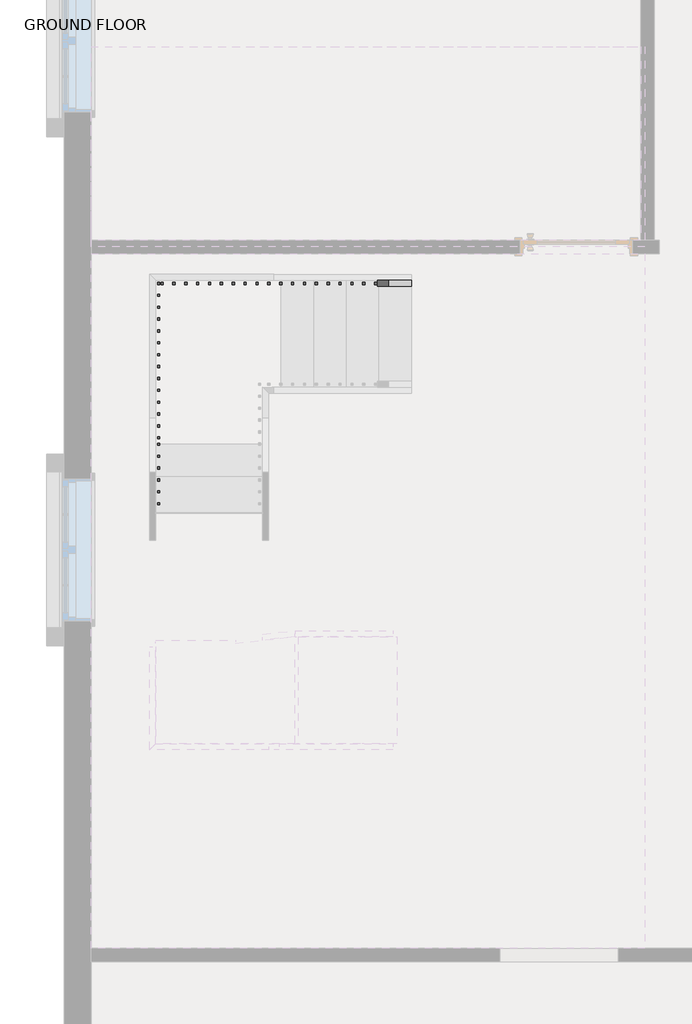
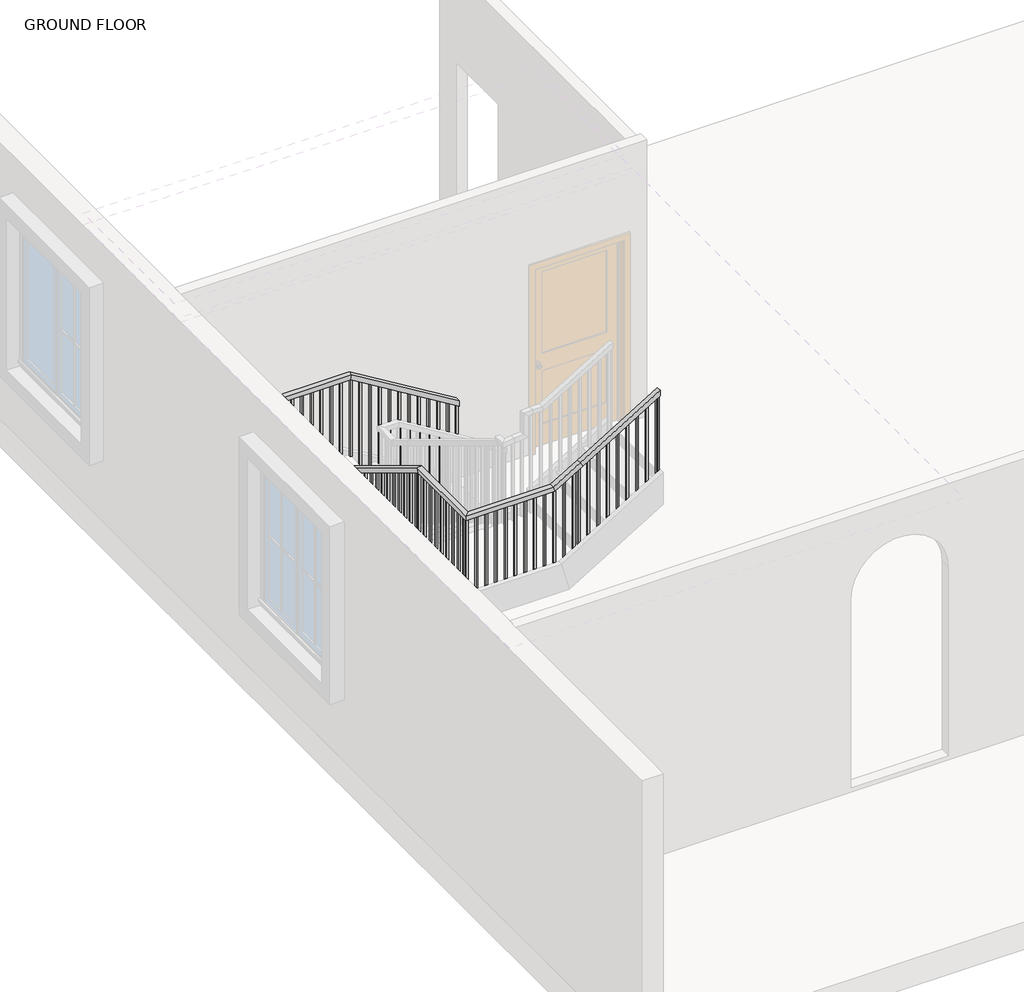
# One storey, part 2 of 4: 1 railing.
"""IFC4 building model written with IfcOpenShell, lengths in millimetres."""

from ifc_helpers import new_model, si_unit, frame, origin, place, context, project, spatial, polyline, outline, extrude, faceted_brep, element, save

model = new_model("IFC4")

# Units and contexts
model_context = context("Model", 3, world=origin())
ifc_project = project(units=[si_unit("LENGTHUNIT", "METRE", prefix="MILLI")], contexts=[model_context])

# Site, building, storey
site = spatial("IfcSite", under=ifc_project)
building = spatial("IfcBuilding", under=site)
storey = spatial("IfcBuildingStorey", under=building, Name="GROUND FLOOR", Elevation=304.8)

# Railing
placement = place(None, origin())
element("IfcRailing", 1, ObjectType="Handrail - Rectangular", at=placement, inside=storey, context=model_context, shape_type="SolidModel", body=[
    faceted_brep([(-9079.7156858, 994.3115003, 1388.5333333), (-9079.7156858, 994.3115003, 1329.1318731), (-9079.7156858, 1045.1115003, 1329.1318731), (-9079.7156858, 1045.1115003, 1388.5333333), (-10197.3156858, 994.3115003, 2065.8666667), (-10211.5080953, 994.3115003, 2015.0666667), (-10211.5080953, 1045.1115003, 2015.0666667), (-10197.3156858, 1045.1115003, 2065.8666667), (-11217.3522729, 994.3115003, 2065.8666667), (-11217.3522729, 994.3115003, 2015.0666667), (-11268.1522729, 1045.1115003, 2015.0666667), (-11268.1522729, 1045.1115003, 2065.8666667), (-11217.3522729, -76.9993654, 2065.8666667), (-11217.3522729, -91.1917748, 2015.0666667), (-11268.1522729, -91.1917748, 2015.0666667), (-11268.1522729, -76.9993654, 2065.8666667), (-11217.3522729, -356.3993654, 2235.2), (-11217.3522729, -382.7290926, 2191.7559502), (-11268.1522729, -382.7290926, 2191.7559502), (-11268.1522729, -356.3993654, 2235.2), (-11217.3522729, -2032.7993654, 3251.2), (-11217.3522729, -2046.9917748, 3200.4), (-11268.1522729, -2046.9917748, 3200.4), (-11268.1522729, -2032.7993654, 3251.2), (-11217.3522729, -2865.2844117, 3251.2), (-11217.3522729, -2865.2844117, 3200.4), (-11268.1522729, -2916.0844117, 3200.4), (-11268.1522729, -2916.0844117, 3251.2), (-10353.7522729, -2865.2844117, 3251.2), (-10339.5598635, -2865.2844117, 3200.4), (-10339.5598635, -2916.0844117, 3200.4), (-10353.7522729, -2916.0844117, 3251.2), (-10074.3522729, -2865.2844117, 3420.5333333), (-10048.0225457, -2865.2844117, 3377.0892835), (-10048.0225457, -2916.0844117, 3377.0892835), (-10074.3522729, -2916.0844117, 3420.5333333), (-9236.1522729, -2865.2844117, 3928.5333333), (-9236.1522729, -2916.0844117, 3928.5333333), (-9236.1522729, -2916.0844117, 3869.1318731), (-9236.1522729, -2865.2844117, 3869.1318731)], [[[0, 1, 2, 3]], [[1, 0, 4, 5]], [[2, 1, 5, 6]], [[3, 2, 6, 7]], [[0, 3, 7, 4]], [[5, 4, 8, 9]], [[6, 5, 9, 10]], [[7, 6, 10, 11]], [[4, 7, 11, 8]], [[9, 8, 12, 13]], [[10, 9, 13, 14]], [[11, 10, 14, 15]], [[8, 11, 15, 12]], [[13, 12, 16, 17]], [[14, 13, 17, 18]], [[15, 14, 18, 19]], [[12, 15, 19, 16]], [[17, 16, 20, 21]], [[18, 17, 21, 22]], [[19, 18, 22, 23]], [[16, 19, 23, 20]], [[21, 20, 24, 25]], [[22, 21, 25, 26]], [[23, 22, 26, 27]], [[20, 23, 27, 24]], [[25, 24, 28, 29]], [[26, 25, 29, 30]], [[27, 26, 30, 31]], [[24, 27, 31, 28]], [[29, 28, 32, 33]], [[30, 29, 33, 34]], [[31, 30, 34, 35]], [[28, 31, 35, 32]], [[36, 37, 38, 39]], [[33, 32, 36, 39]], [[34, 33, 39, 38]], [[35, 34, 38, 37]], [[32, 35, 37, 36]]]),
    extrude(outline(polyline([(3859.510661, -9252.0272729), (3847.9652064, -9271.0772729), (2844.8, -9271.0772729), (2844.8, -9252.0272729), (3859.510661, -9252.0272729)])), frame((0.0, -2900.2094117, 0.0), z_axis=(0.0, 1.0, 0.0), x_axis=(0.0, 0.0, 1.0)), (0.0, 0.0, 1.0), 19.05),
    extrude(outline(polyline([(3797.9349034, -9353.6272729), (3786.3894488, -9372.6772729), (2844.8, -9372.6772729), (2844.8, -9353.6272729), (3797.9349034, -9353.6272729)])), frame((0.0, -2900.2094117, 0.0), z_axis=(0.0, 1.0, 0.0), x_axis=(0.0, 0.0, 1.0)), (0.0, 0.0, 1.0), 19.05),
    extrude(outline(polyline([(3736.3591458, -9455.2272729), (3724.8136913, -9474.2772729), (2844.8, -9474.2772729), (2844.8, -9455.2272729), (3736.3591458, -9455.2272729)])), frame((0.0, -2900.2094117, 0.0), z_axis=(0.0, 1.0, 0.0), x_axis=(0.0, 0.0, 1.0)), (0.0, 0.0, 1.0), 19.05),
    extrude(outline(polyline([(3674.7833882, -9556.8272729), (3663.2379337, -9575.8772729), (2675.4666667, -9575.8772729), (2675.4666667, -9556.8272729), (3674.7833882, -9556.8272729)])), frame((0.0, -2900.2094117, 0.0), z_axis=(0.0, 1.0, 0.0), x_axis=(0.0, 0.0, 1.0)), (0.0, 0.0, 1.0), 19.05),
    extrude(outline(polyline([(3613.2076307, -9658.4272729), (3601.6621761, -9677.4772729), (2675.4666667, -9677.4772729), (2675.4666667, -9658.4272729), (3613.2076307, -9658.4272729)])), frame((0.0, -2900.2094117, 0.0), z_axis=(0.0, 1.0, 0.0), x_axis=(0.0, 0.0, 1.0)), (0.0, 0.0, 1.0), 19.05),
    extrude(outline(polyline([(3551.6960801, -9760.0272729), (3540.0063073, -9779.0772729), (2675.4666667, -9779.0772729), (2675.4666667, -9760.0272729), (3551.6960801, -9760.0272729)])), frame((0.0, -2900.2094117, 0.0), z_axis=(0.0, 1.0, 0.0), x_axis=(0.0, 0.0, 1.0)), (0.0, 0.0, 1.0), 19.05),
    extrude(outline(polyline([(3490.0561155, -9861.6272729), (3478.510661, -9880.6772729), (2506.1333333, -9880.6772729), (2506.1333333, -9861.6272729), (3490.0561155, -9861.6272729)])), frame((0.0, -2900.2094117, 0.0), z_axis=(0.0, 1.0, 0.0), x_axis=(0.0, 0.0, 1.0)), (0.0, 0.0, 1.0), 19.05),
    extrude(outline(polyline([(3428.4803579, -9963.2272729), (3416.9349034, -9982.2772729), (2506.1333333, -9982.2772729), (2506.1333333, -9963.2272729), (3428.4803579, -9963.2272729)])), frame((0.0, -2900.2094117, 0.0), z_axis=(0.0, 1.0, 0.0), x_axis=(0.0, 0.0, 1.0)), (0.0, 0.0, 1.0), 19.05),
    extrude(outline(polyline([(3336.1167216, -10115.6272729), (3324.571267, -10134.6772729), (2336.8, -10134.6772729), (2336.8, -10115.6272729), (3336.1167216, -10115.6272729)])), frame((0.0, -2900.2094117, 0.0), z_axis=(0.0, 1.0, 0.0), x_axis=(0.0, 0.0, 1.0)), (0.0, 0.0, 1.0), 19.05),
    extrude(outline(polyline([(3274.540964, -10217.2272729), (3262.9955094, -10236.2772729), (2336.8, -10236.2772729), (2336.8, -10217.2272729), (3274.540964, -10217.2272729)])), frame((0.0, -2900.2094117, 0.0), z_axis=(0.0, 1.0, 0.0), x_axis=(0.0, 0.0, 1.0)), (0.0, 0.0, 1.0), 19.05),
    extrude(outline(polyline([(3213.0294134, -10318.8272729), (3201.3396407, -10337.8772729), (2336.8, -10337.8772729), (2336.8, -10318.8272729), (3213.0294134, -10318.8272729)])), frame((0.0, -2900.2094117, 0.0), z_axis=(0.0, 1.0, 0.0), x_axis=(0.0, 0.0, 1.0)), (0.0, 0.0, 1.0), 19.05),
    extrude(outline(polyline([(-10439.4772729, -2900.2094117), (-10439.4772729, -2881.1594117), (-10420.4272729, -2881.1594117), (-10420.4272729, -2900.2094117), (-10439.4772729, -2900.2094117)])), frame((0.0, 0.0, 2336.8), z_axis=(0.0, 0.0, 1.0), x_axis=(1.0, 0.0, 0.0)), (0.0, 0.0, 1.0), 863.6),
    extrude(outline(polyline([(-10541.0772729, -2900.2094117), (-10541.0772729, -2881.1594117), (-10522.0272729, -2881.1594117), (-10522.0272729, -2900.2094117), (-10541.0772729, -2900.2094117)])), frame((0.0, 0.0, 2336.8), z_axis=(0.0, 0.0, 1.0), x_axis=(1.0, 0.0, 0.0)), (0.0, 0.0, 1.0), 863.6),
    extrude(outline(polyline([(-10642.6772729, -2900.2094117), (-10642.6772729, -2881.1594117), (-10623.6272729, -2881.1594117), (-10623.6272729, -2900.2094117), (-10642.6772729, -2900.2094117)])), frame((0.0, 0.0, 2336.8), z_axis=(0.0, 0.0, 1.0), x_axis=(1.0, 0.0, 0.0)), (0.0, 0.0, 1.0), 863.6),
    extrude(outline(polyline([(-10744.2772729, -2900.2094117), (-10744.2772729, -2881.1594117), (-10725.2272729, -2881.1594117), (-10725.2272729, -2900.2094117), (-10744.2772729, -2900.2094117)])), frame((0.0, 0.0, 2336.8), z_axis=(0.0, 0.0, 1.0), x_axis=(1.0, 0.0, 0.0)), (0.0, 0.0, 1.0), 863.6),
    extrude(outline(polyline([(-10845.8772729, -2900.2094117), (-10845.8772729, -2881.1594117), (-10826.8272729, -2881.1594117), (-10826.8272729, -2900.2094117), (-10845.8772729, -2900.2094117)])), frame((0.0, 0.0, 2336.8), z_axis=(0.0, 0.0, 1.0), x_axis=(1.0, 0.0, 0.0)), (0.0, 0.0, 1.0), 863.6),
    extrude(outline(polyline([(-10947.4772729, -2900.2094117), (-10947.4772729, -2881.1594117), (-10928.4272729, -2881.1594117), (-10928.4272729, -2900.2094117), (-10947.4772729, -2900.2094117)])), frame((0.0, 0.0, 2336.8), z_axis=(0.0, 0.0, 1.0), x_axis=(1.0, 0.0, 0.0)), (0.0, 0.0, 1.0), 863.6),
    extrude(outline(polyline([(-11049.0772729, -2900.2094117), (-11049.0772729, -2881.1594117), (-11030.0272729, -2881.1594117), (-11030.0272729, -2900.2094117), (-11049.0772729, -2900.2094117)])), frame((0.0, 0.0, 2336.8), z_axis=(0.0, 0.0, 1.0), x_axis=(1.0, 0.0, 0.0)), (0.0, 0.0, 1.0), 863.6),
    extrude(outline(polyline([(-11150.6772729, -2900.2094117), (-11150.6772729, -2881.1594117), (-11131.6272729, -2881.1594117), (-11131.6272729, -2900.2094117), (-11150.6772729, -2900.2094117)])), frame((0.0, 0.0, 2336.8), z_axis=(0.0, 0.0, 1.0), x_axis=(1.0, 0.0, 0.0)), (0.0, 0.0, 1.0), 863.6),
    extrude(outline(polyline([(-11252.2772729, -2836.0743654), (-11233.2272729, -2836.0743654), (-11233.2272729, -2855.1243654), (-11252.2772729, -2855.1243654), (-11252.2772729, -2836.0743654)])), frame((0.0, 0.0, 2336.8), z_axis=(0.0, 0.0, 1.0), x_axis=(1.0, 0.0, 0.0)), (0.0, 0.0, 1.0), 863.6),
    extrude(outline(polyline([(-11252.2772729, -2734.4743654), (-11233.2272729, -2734.4743654), (-11233.2272729, -2753.5243654), (-11252.2772729, -2753.5243654), (-11252.2772729, -2734.4743654)])), frame((0.0, 0.0, 2336.8), z_axis=(0.0, 0.0, 1.0), x_axis=(1.0, 0.0, 0.0)), (0.0, 0.0, 1.0), 863.6),
    extrude(outline(polyline([(-11252.2772729, -2632.8743654), (-11233.2272729, -2632.8743654), (-11233.2272729, -2651.9243654), (-11252.2772729, -2651.9243654), (-11252.2772729, -2632.8743654)])), frame((0.0, 0.0, 2336.8), z_axis=(0.0, 0.0, 1.0), x_axis=(1.0, 0.0, 0.0)), (0.0, 0.0, 1.0), 863.6),
    extrude(outline(polyline([(-11252.2772729, -2531.2743654), (-11233.2272729, -2531.2743654), (-11233.2272729, -2550.3243654), (-11252.2772729, -2550.3243654), (-11252.2772729, -2531.2743654)])), frame((0.0, 0.0, 2336.8), z_axis=(0.0, 0.0, 1.0), x_axis=(1.0, 0.0, 0.0)), (0.0, 0.0, 1.0), 863.6),
    extrude(outline(polyline([(-11252.2772729, -2429.6743654), (-11233.2272729, -2429.6743654), (-11233.2272729, -2448.7243654), (-11252.2772729, -2448.7243654), (-11252.2772729, -2429.6743654)])), frame((0.0, 0.0, 2336.8), z_axis=(0.0, 0.0, 1.0), x_axis=(1.0, 0.0, 0.0)), (0.0, 0.0, 1.0), 863.6),
    extrude(outline(polyline([(-11252.2772729, -2328.0743654), (-11233.2272729, -2328.0743654), (-11233.2272729, -2347.1243654), (-11252.2772729, -2347.1243654), (-11252.2772729, -2328.0743654)])), frame((0.0, 0.0, 2336.8), z_axis=(0.0, 0.0, 1.0), x_axis=(1.0, 0.0, 0.0)), (0.0, 0.0, 1.0), 863.6),
    extrude(outline(polyline([(-11252.2772729, -2226.4743654), (-11233.2272729, -2226.4743654), (-11233.2272729, -2245.5243654), (-11252.2772729, -2245.5243654), (-11252.2772729, -2226.4743654)])), frame((0.0, 0.0, 2336.8), z_axis=(0.0, 0.0, 1.0), x_axis=(1.0, 0.0, 0.0)), (0.0, 0.0, 1.0), 863.6),
    extrude(outline(polyline([(-11252.2772729, -2124.8743654), (-11233.2272729, -2124.8743654), (-11233.2272729, -2143.9243654), (-11252.2772729, -2143.9243654), (-11252.2772729, -2124.8743654)])), frame((0.0, 0.0, 2336.8), z_axis=(0.0, 0.0, 1.0), x_axis=(1.0, 0.0, 0.0)), (0.0, 0.0, 1.0), 863.6),
    extrude(outline(polyline([(-1991.5243654, 3166.7833882), (-1972.4743654, 3155.2379337), (-1972.4743654, 2167.4666667), (-1991.5243654, 2167.4666667), (-1991.5243654, 3166.7833882)])), frame((-11252.2772729, 0.0, 0.0), z_axis=(1.0, 0.0, 0.0), x_axis=(0.0, 1.0, 0.0)), (0.0, 0.0, 1.0), 19.05),
    extrude(outline(polyline([(-1889.9243654, 3105.2076307), (-1870.8743654, 3093.6621761), (-1870.8743654, 2167.4666667), (-1889.9243654, 2167.4666667), (-1889.9243654, 3105.2076307)])), frame((-11252.2772729, 0.0, 0.0), z_axis=(1.0, 0.0, 0.0), x_axis=(0.0, 1.0, 0.0)), (0.0, 0.0, 1.0), 19.05),
    extrude(outline(polyline([(-1788.3243654, 3043.6960801), (-1769.2743654, 3032.0063073), (-1769.2743654, 2167.4666667), (-1788.3243654, 2167.4666667), (-1788.3243654, 3043.6960801)])), frame((-11252.2772729, 0.0, 0.0), z_axis=(1.0, 0.0, 0.0), x_axis=(0.0, 1.0, 0.0)), (0.0, 0.0, 1.0), 19.05),
    extrude(outline(polyline([(-1686.7243654, 2982.0561155), (-1667.6743654, 2970.510661), (-1667.6743654, 1998.1333333), (-1686.7243654, 1998.1333333), (-1686.7243654, 2982.0561155)])), frame((-11252.2772729, 0.0, 0.0), z_axis=(1.0, 0.0, 0.0), x_axis=(0.0, 1.0, 0.0)), (0.0, 0.0, 1.0), 19.05),
    extrude(outline(polyline([(-1585.1243654, 2920.4803579), (-1566.0743654, 2908.9349034), (-1566.0743654, 1998.1333333), (-1585.1243654, 1998.1333333), (-1585.1243654, 2920.4803579)])), frame((-11252.2772729, 0.0, 0.0), z_axis=(1.0, 0.0, 0.0), x_axis=(0.0, 1.0, 0.0)), (0.0, 0.0, 1.0), 19.05),
    extrude(outline(polyline([(-1483.5243654, 2858.9046004), (-1464.4743654, 2847.3591458), (-1464.4743654, 1998.1333333), (-1483.5243654, 1998.1333333), (-1483.5243654, 2858.9046004)])), frame((-11252.2772729, 0.0, 0.0), z_axis=(1.0, 0.0, 0.0), x_axis=(0.0, 1.0, 0.0)), (0.0, 0.0, 1.0), 19.05),
    extrude(outline(polyline([(-1381.9243654, 2797.3288428), (-1362.8743654, 2785.7833882), (-1362.8743654, 1828.8), (-1381.9243654, 1828.8), (-1381.9243654, 2797.3288428)])), frame((-11252.2772729, 0.0, 0.0), z_axis=(1.0, 0.0, 0.0), x_axis=(0.0, 1.0, 0.0)), (0.0, 0.0, 1.0), 19.05),
    extrude(outline(polyline([(-1280.3243654, 2735.7530852), (-1261.2743654, 2724.2076307), (-1261.2743654, 1828.8), (-1280.3243654, 1828.8), (-1280.3243654, 2735.7530852)])), frame((-11252.2772729, 0.0, 0.0), z_axis=(1.0, 0.0, 0.0), x_axis=(0.0, 1.0, 0.0)), (0.0, 0.0, 1.0), 19.05),
    extrude(outline(polyline([(-1178.7243654, 2674.1773276), (-1159.6743654, 2662.6318731), (-1159.6743654, 1659.4666667), (-1178.7243654, 1659.4666667), (-1178.7243654, 2674.1773276)])), frame((-11252.2772729, 0.0, 0.0), z_axis=(1.0, 0.0, 0.0), x_axis=(0.0, 1.0, 0.0)), (0.0, 0.0, 1.0), 19.05),
    extrude(outline(polyline([(-1077.1243654, 2612.60157), (-1058.0743654, 2601.0561155), (-1058.0743654, 1659.4666667), (-1077.1243654, 1659.4666667), (-1077.1243654, 2612.60157)])), frame((-11252.2772729, 0.0, 0.0), z_axis=(1.0, 0.0, 0.0), x_axis=(0.0, 1.0, 0.0)), (0.0, 0.0, 1.0), 19.05),
    extrude(outline(polyline([(-975.5243654, 2551.0258125), (-956.4743654, 2539.4803579), (-956.4743654, 1659.4666667), (-975.5243654, 1659.4666667), (-975.5243654, 2551.0258125)])), frame((-11252.2772729, 0.0, 0.0), z_axis=(1.0, 0.0, 0.0), x_axis=(0.0, 1.0, 0.0)), (0.0, 0.0, 1.0), 19.05),
    extrude(outline(polyline([(-873.9243654, 2489.4500549), (-854.8743654, 2477.9046004), (-854.8743654, 1490.1333333), (-873.9243654, 1490.1333333), (-873.9243654, 2489.4500549)])), frame((-11252.2772729, 0.0, 0.0), z_axis=(1.0, 0.0, 0.0), x_axis=(0.0, 1.0, 0.0)), (0.0, 0.0, 1.0), 19.05),
    extrude(outline(polyline([(-772.3243654, 2427.8742973), (-753.2743654, 2416.3288428), (-753.2743654, 1490.1333333), (-772.3243654, 1490.1333333), (-772.3243654, 2427.8742973)])), frame((-11252.2772729, 0.0, 0.0), z_axis=(1.0, 0.0, 0.0), x_axis=(0.0, 1.0, 0.0)), (0.0, 0.0, 1.0), 19.05),
    extrude(outline(polyline([(-670.7243654, 2366.3627467), (-651.6743654, 2354.672974), (-651.6743654, 1490.1333333), (-670.7243654, 1490.1333333), (-670.7243654, 2366.3627467)])), frame((-11252.2772729, 0.0, 0.0), z_axis=(1.0, 0.0, 0.0), x_axis=(0.0, 1.0, 0.0)), (0.0, 0.0, 1.0), 19.05),
    extrude(outline(polyline([(-569.1243654, 2304.7227822), (-550.0743654, 2293.1773276), (-550.0743654, 1320.8), (-569.1243654, 1320.8), (-569.1243654, 2304.7227822)])), frame((-11252.2772729, 0.0, 0.0), z_axis=(1.0, 0.0, 0.0), x_axis=(0.0, 1.0, 0.0)), (0.0, 0.0, 1.0), 19.05),
    extrude(outline(polyline([(-467.5243654, 2243.1470246), (-448.4743654, 2231.60157), (-448.4743654, 1320.8), (-467.5243654, 1320.8), (-467.5243654, 2243.1470246)])), frame((-11252.2772729, 0.0, 0.0), z_axis=(1.0, 0.0, 0.0), x_axis=(0.0, 1.0, 0.0)), (0.0, 0.0, 1.0), 19.05),
    extrude(outline(polyline([(-310.6134997, 2148.0495303), (-291.5634997, 2136.5040757), (-291.5634997, 1151.4666667), (-310.6134997, 1151.4666667), (-310.6134997, 2148.0495303)])), frame((-11252.2772729, 0.0, 0.0), z_axis=(1.0, 0.0, 0.0), x_axis=(0.0, 1.0, 0.0)), (0.0, 0.0, 1.0), 19.05),
    extrude(outline(polyline([(-209.0134997, 2086.4737727), (-189.9634997, 2074.9283181), (-189.9634997, 1151.4666667), (-209.0134997, 1151.4666667), (-209.0134997, 2086.4737727)])), frame((-11252.2772729, 0.0, 0.0), z_axis=(1.0, 0.0, 0.0), x_axis=(0.0, 1.0, 0.0)), (0.0, 0.0, 1.0), 19.05),
    extrude(outline(polyline([(-107.4134997, 2024.9280489), (-88.3634997, 2013.2382761), (-88.3634997, 1151.4666667), (-107.4134997, 1151.4666667), (-107.4134997, 2024.9280489)])), frame((-11252.2772729, 0.0, 0.0), z_axis=(1.0, 0.0, 0.0), x_axis=(0.0, 1.0, 0.0)), (0.0, 0.0, 1.0), 19.05),
    extrude(outline(polyline([(-11252.2772729, 13.2365003), (-11233.2272729, 13.2365003), (-11233.2272729, -5.8134997), (-11252.2772729, -5.8134997), (-11252.2772729, 13.2365003)])), frame((0.0, 0.0, 1151.4666667), z_axis=(0.0, 0.0, 1.0), x_axis=(1.0, 0.0, 0.0)), (0.0, 0.0, 1.0), 863.6),
    extrude(outline(polyline([(-11252.2772729, 114.8365003), (-11233.2272729, 114.8365003), (-11233.2272729, 95.7865003), (-11252.2772729, 95.7865003), (-11252.2772729, 114.8365003)])), frame((0.0, 0.0, 1151.4666667), z_axis=(0.0, 0.0, 1.0), x_axis=(1.0, 0.0, 0.0)), (0.0, 0.0, 1.0), 863.6),
    extrude(outline(polyline([(-11252.2772729, 216.4365003), (-11233.2272729, 216.4365003), (-11233.2272729, 197.3865003), (-11252.2772729, 197.3865003), (-11252.2772729, 216.4365003)])), frame((0.0, 0.0, 1151.4666667), z_axis=(0.0, 0.0, 1.0), x_axis=(1.0, 0.0, 0.0)), (0.0, 0.0, 1.0), 863.6),
    extrude(outline(polyline([(-11252.2772729, 318.0365003), (-11233.2272729, 318.0365003), (-11233.2272729, 298.9865003), (-11252.2772729, 298.9865003), (-11252.2772729, 318.0365003)])), frame((0.0, 0.0, 1151.4666667), z_axis=(0.0, 0.0, 1.0), x_axis=(1.0, 0.0, 0.0)), (0.0, 0.0, 1.0), 863.6),
    extrude(outline(polyline([(-11252.2772729, 419.6365003), (-11233.2272729, 419.6365003), (-11233.2272729, 400.5865003), (-11252.2772729, 400.5865003), (-11252.2772729, 419.6365003)])), frame((0.0, 0.0, 1151.4666667), z_axis=(0.0, 0.0, 1.0), x_axis=(1.0, 0.0, 0.0)), (0.0, 0.0, 1.0), 863.6),
    extrude(outline(polyline([(-11252.2772729, 521.2365003), (-11233.2272729, 521.2365003), (-11233.2272729, 502.1865003), (-11252.2772729, 502.1865003), (-11252.2772729, 521.2365003)])), frame((0.0, 0.0, 1151.4666667), z_axis=(0.0, 0.0, 1.0), x_axis=(1.0, 0.0, 0.0)), (0.0, 0.0, 1.0), 863.6),
    extrude(outline(polyline([(-11252.2772729, 622.8365003), (-11233.2272729, 622.8365003), (-11233.2272729, 603.7865003), (-11252.2772729, 603.7865003), (-11252.2772729, 622.8365003)])), frame((0.0, 0.0, 1151.4666667), z_axis=(0.0, 0.0, 1.0), x_axis=(1.0, 0.0, 0.0)), (0.0, 0.0, 1.0), 863.6),
    extrude(outline(polyline([(-11252.2772729, 724.4365003), (-11233.2272729, 724.4365003), (-11233.2272729, 705.3865003), (-11252.2772729, 705.3865003), (-11252.2772729, 724.4365003)])), frame((0.0, 0.0, 1151.4666667), z_axis=(0.0, 0.0, 1.0), x_axis=(1.0, 0.0, 0.0)), (0.0, 0.0, 1.0), 863.6),
    extrude(outline(polyline([(-11252.2772729, 826.0365003), (-11233.2272729, 826.0365003), (-11233.2272729, 806.9865003), (-11252.2772729, 806.9865003), (-11252.2772729, 826.0365003)])), frame((0.0, 0.0, 1151.4666667), z_axis=(0.0, 0.0, 1.0), x_axis=(1.0, 0.0, 0.0)), (0.0, 0.0, 1.0), 863.6),
    extrude(outline(polyline([(-11252.2772729, 927.6365003), (-11233.2272729, 927.6365003), (-11233.2272729, 908.5865003), (-11252.2772729, 908.5865003), (-11252.2772729, 927.6365003)])), frame((0.0, 0.0, 1151.4666667), z_axis=(0.0, 0.0, 1.0), x_axis=(1.0, 0.0, 0.0)), (0.0, 0.0, 1.0), 863.6),
    extrude(outline(polyline([(-11203.7906858, 1029.2365003), (-11203.7906858, 1010.1865003), (-11222.8406858, 1010.1865003), (-11222.8406858, 1029.2365003), (-11203.7906858, 1029.2365003)])), frame((0.0, 0.0, 1151.4666667), z_axis=(0.0, 0.0, 1.0), x_axis=(1.0, 0.0, 0.0)), (0.0, 0.0, 1.0), 863.6),
    extrude(outline(polyline([(-11102.1906858, 1029.2365003), (-11102.1906858, 1010.1865003), (-11121.2406858, 1010.1865003), (-11121.2406858, 1029.2365003), (-11102.1906858, 1029.2365003)])), frame((0.0, 0.0, 1151.4666667), z_axis=(0.0, 0.0, 1.0), x_axis=(1.0, 0.0, 0.0)), (0.0, 0.0, 1.0), 863.6),
    extrude(outline(polyline([(-11000.5906858, 1029.2365003), (-11000.5906858, 1010.1865003), (-11019.6406858, 1010.1865003), (-11019.6406858, 1029.2365003), (-11000.5906858, 1029.2365003)])), frame((0.0, 0.0, 1151.4666667), z_axis=(0.0, 0.0, 1.0), x_axis=(1.0, 0.0, 0.0)), (0.0, 0.0, 1.0), 863.6),
    extrude(outline(polyline([(-10898.9906858, 1029.2365003), (-10898.9906858, 1010.1865003), (-10918.0406858, 1010.1865003), (-10918.0406858, 1029.2365003), (-10898.9906858, 1029.2365003)])), frame((0.0, 0.0, 1151.4666667), z_axis=(0.0, 0.0, 1.0), x_axis=(1.0, 0.0, 0.0)), (0.0, 0.0, 1.0), 863.6),
    extrude(outline(polyline([(-10797.3906858, 1029.2365003), (-10797.3906858, 1010.1865003), (-10816.4406858, 1010.1865003), (-10816.4406858, 1029.2365003), (-10797.3906858, 1029.2365003)])), frame((0.0, 0.0, 1151.4666667), z_axis=(0.0, 0.0, 1.0), x_axis=(1.0, 0.0, 0.0)), (0.0, 0.0, 1.0), 863.6),
    extrude(outline(polyline([(-10695.7906858, 1029.2365003), (-10695.7906858, 1010.1865003), (-10714.8406858, 1010.1865003), (-10714.8406858, 1029.2365003), (-10695.7906858, 1029.2365003)])), frame((0.0, 0.0, 1151.4666667), z_axis=(0.0, 0.0, 1.0), x_axis=(1.0, 0.0, 0.0)), (0.0, 0.0, 1.0), 863.6),
    extrude(outline(polyline([(-10594.1906858, 1029.2365003), (-10594.1906858, 1010.1865003), (-10613.2406858, 1010.1865003), (-10613.2406858, 1029.2365003), (-10594.1906858, 1029.2365003)])), frame((0.0, 0.0, 1151.4666667), z_axis=(0.0, 0.0, 1.0), x_axis=(1.0, 0.0, 0.0)), (0.0, 0.0, 1.0), 863.6),
    extrude(outline(polyline([(-10492.5906858, 1029.2365003), (-10492.5906858, 1010.1865003), (-10511.6406858, 1010.1865003), (-10511.6406858, 1029.2365003), (-10492.5906858, 1029.2365003)])), frame((0.0, 0.0, 1151.4666667), z_axis=(0.0, 0.0, 1.0), x_axis=(1.0, 0.0, 0.0)), (0.0, 0.0, 1.0), 863.6),
    extrude(outline(polyline([(-10390.9906858, 1029.2365003), (-10390.9906858, 1010.1865003), (-10410.0406858, 1010.1865003), (-10410.0406858, 1029.2365003), (-10390.9906858, 1029.2365003)])), frame((0.0, 0.0, 1151.4666667), z_axis=(0.0, 0.0, 1.0), x_axis=(1.0, 0.0, 0.0)), (0.0, 0.0, 1.0), 863.6),
    extrude(outline(polyline([(-10289.3906858, 1029.2365003), (-10289.3906858, 1010.1865003), (-10308.4406858, 1010.1865003), (-10308.4406858, 1029.2365003), (-10289.3906858, 1029.2365003)])), frame((0.0, 0.0, 1151.4666667), z_axis=(0.0, 0.0, 1.0), x_axis=(1.0, 0.0, 0.0)), (0.0, 0.0, 1.0), 863.6),
    extrude(outline(polyline([(1939.1167216, -10086.1906858), (1950.6621761, -10105.2406858), (982.1333333, -10105.2406858), (982.1333333, -10086.1906858), (1939.1167216, -10086.1906858)])), frame((0.0, 1010.1865003, 0.0), z_axis=(0.0, 1.0, 0.0), x_axis=(0.0, 0.0, 1.0)), (0.0, 0.0, 1.0), 19.05),
    extrude(outline(polyline([(1877.540964, -9984.5906858), (1889.0864185, -10003.6406858), (982.1333333, -10003.6406858), (982.1333333, -9984.5906858), (1877.540964, -9984.5906858)])), frame((0.0, 1010.1865003, 0.0), z_axis=(0.0, 1.0, 0.0), x_axis=(0.0, 0.0, 1.0)), (0.0, 0.0, 1.0), 19.05),
    extrude(outline(polyline([(1815.9652064, -9882.9906858), (1827.510661, -9902.0406858), (812.8, -9902.0406858), (812.8, -9882.9906858), (1815.9652064, -9882.9906858)])), frame((0.0, 1010.1865003, 0.0), z_axis=(0.0, 1.0, 0.0), x_axis=(0.0, 0.0, 1.0)), (0.0, 0.0, 1.0), 19.05),
    extrude(outline(polyline([(1754.3894488, -9781.3906858), (1765.9349034, -9800.4406858), (812.8, -9800.4406858), (812.8, -9781.3906858), (1754.3894488, -9781.3906858)])), frame((0.0, 1010.1865003, 0.0), z_axis=(0.0, 1.0, 0.0), x_axis=(0.0, 0.0, 1.0)), (0.0, 0.0, 1.0), 19.05),
    extrude(outline(polyline([(1692.8136913, -9679.7906858), (1704.3591458, -9698.8406858), (812.8, -9698.8406858), (812.8, -9679.7906858), (1692.8136913, -9679.7906858)])), frame((0.0, 1010.1865003, 0.0), z_axis=(0.0, 1.0, 0.0), x_axis=(0.0, 0.0, 1.0)), (0.0, 0.0, 1.0), 19.05),
    extrude(outline(polyline([(1631.2379337, -9578.1906858), (1642.7833882, -9597.2406858), (643.4666667, -9597.2406858), (643.4666667, -9578.1906858), (1631.2379337, -9578.1906858)])), frame((0.0, 1010.1865003, 0.0), z_axis=(0.0, 1.0, 0.0), x_axis=(0.0, 0.0, 1.0)), (0.0, 0.0, 1.0), 19.05),
    extrude(outline(polyline([(1569.6621761, -9476.5906858), (1581.2076307, -9495.6406858), (643.4666667, -9495.6406858), (643.4666667, -9476.5906858), (1569.6621761, -9476.5906858)])), frame((0.0, 1010.1865003, 0.0), z_axis=(0.0, 1.0, 0.0), x_axis=(0.0, 0.0, 1.0)), (0.0, 0.0, 1.0), 19.05),
    extrude(outline(polyline([(1508.0063073, -9374.9906858), (1519.6960801, -9394.0406858), (643.4666667, -9394.0406858), (643.4666667, -9374.9906858), (1508.0063073, -9374.9906858)])), frame((0.0, 1010.1865003, 0.0), z_axis=(0.0, 1.0, 0.0), x_axis=(0.0, 0.0, 1.0)), (0.0, 0.0, 1.0), 19.05),
    extrude(outline(polyline([(1446.510661, -9273.3906858), (1458.0561155, -9292.4406858), (474.1333333, -9292.4406858), (474.1333333, -9273.3906858), (1446.510661, -9273.3906858)])), frame((0.0, 1010.1865003, 0.0), z_axis=(0.0, 1.0, 0.0), x_axis=(0.0, 0.0, 1.0)), (0.0, 0.0, 1.0), 19.05),
    extrude(outline(polyline([(1384.9349034, -9171.7906858), (1396.4803579, -9190.8406858), (474.1333333, -9190.8406858), (474.1333333, -9171.7906858), (1384.9349034, -9171.7906858)])), frame((0.0, 1010.1865003, 0.0), z_axis=(0.0, 1.0, 0.0), x_axis=(0.0, 0.0, 1.0)), (0.0, 0.0, 1.0), 19.05),
    extrude(outline(polyline([(3366.9046004, -10064.8272729), (3355.3591458, -10083.8772729), (2336.8, -10083.8772729), (2336.8, -10064.8272729), (3366.9046004, -10064.8272729)])), frame((0.0, -2900.2094117, 0.0), z_axis=(0.0, 1.0, 0.0), x_axis=(0.0, 0.0, 1.0)), (0.0, 0.0, 1.0), 19.05),
    extrude(outline(polyline([(-11252.2772729, -2881.1594117), (-11233.2272729, -2881.1594117), (-11233.2272729, -2900.2094117), (-11252.2772729, -2900.2094117), (-11252.2772729, -2881.1594117)])), frame((0.0, 0.0, 2336.8), z_axis=(0.0, 0.0, 1.0), x_axis=(1.0, 0.0, 0.0)), (0.0, 0.0, 1.0), 863.6),
    extrude(outline(polyline([(-2042.3243654, 3197.571267), (-2023.2743654, 3186.0258125), (-2023.2743654, 2336.8), (-2042.3243654, 2336.8), (-2042.3243654, 3197.571267)])), frame((-11252.2772729, 0.0, 0.0), z_axis=(1.0, 0.0, 0.0), x_axis=(0.0, 1.0, 0.0)), (0.0, 0.0, 1.0), 19.05),
    extrude(outline(polyline([(-365.9243654, 2181.571267), (-346.8743654, 2170.0258125), (-346.8743654, 1151.4666667), (-365.9243654, 1151.4666667), (-365.9243654, 2181.571267)])), frame((-11252.2772729, 0.0, 0.0), z_axis=(1.0, 0.0, 0.0), x_axis=(0.0, 1.0, 0.0)), (0.0, 0.0, 1.0), 19.05),
    extrude(outline(polyline([(-11233.2272729, 1029.2365003), (-11233.2272729, 1010.1865003), (-11252.2772729, 1010.1865003), (-11252.2772729, 1029.2365003), (-11233.2272729, 1029.2365003)])), frame((0.0, 0.0, 1151.4666667), z_axis=(0.0, 0.0, 1.0), x_axis=(1.0, 0.0, 0.0)), (0.0, 0.0, 1.0), 863.6),
    extrude(outline(polyline([(2000.6924791, -10187.7906858), (2012.2379337, -10206.8406858), (1151.4666667, -10206.8406858), (1151.4666667, -10187.7906858), (2000.6924791, -10187.7906858)])), frame((0.0, 1010.1865003, 0.0), z_axis=(0.0, 1.0, 0.0), x_axis=(0.0, 0.0, 1.0)), (0.0, 0.0, 1.0), 19.05),
    extrude(outline(polyline([(3869.1318731, -9236.1522729), (3857.5864185, -9255.2022729), (2844.8, -9255.2022729), (2844.8, -9236.1522729), (3869.1318731, -9236.1522729)])), frame((0.0, -2900.2094117, 0.0), z_axis=(0.0, 1.0, 0.0), x_axis=(0.0, 0.0, 1.0)), (0.0, 0.0, 1.0), 19.05),
    extrude(outline(polyline([(1328.9314967, -9079.7156858), (1340.6212695, -9098.7656858), (474.1333333, -9098.7656858), (474.1333333, -9079.7156858), (1328.9314967, -9079.7156858)])), frame((0.0, 1010.1865003, 0.0), z_axis=(0.0, 1.0, 0.0), x_axis=(0.0, 0.0, 1.0)), (0.0, 0.0, 1.0), 19.05),
])

save(model, "model.ifc")

# Revit data of these elements
# Type "Handrail - Rectangular"
#   Assembly Code = "C2010400"
#   built-in parameter 1008612 = 0.0416667 (stored number, unit not read)
#   built-in parameter 1008611 = 0.0416667 (stored number, unit not read)
#   built-in parameter 1008609 = 0.333333 (stored number, unit not read)
#   built-in parameter 1008604 = 0.166667 (stored number, unit not read)
#   built-in parameter 1008603 = 0.166667 (stored number, unit not read)
#   Railing Height = 3' - 0"
#   built-in parameter 1008630 = 2
#   built-in parameter 1008610 = 2
#   built-in parameter 1008618 = Baluster - Square : 3/4"
# Element 1 (IfcRailing, "Handrail - Rectangular")
#   Phase Created = New Construction
